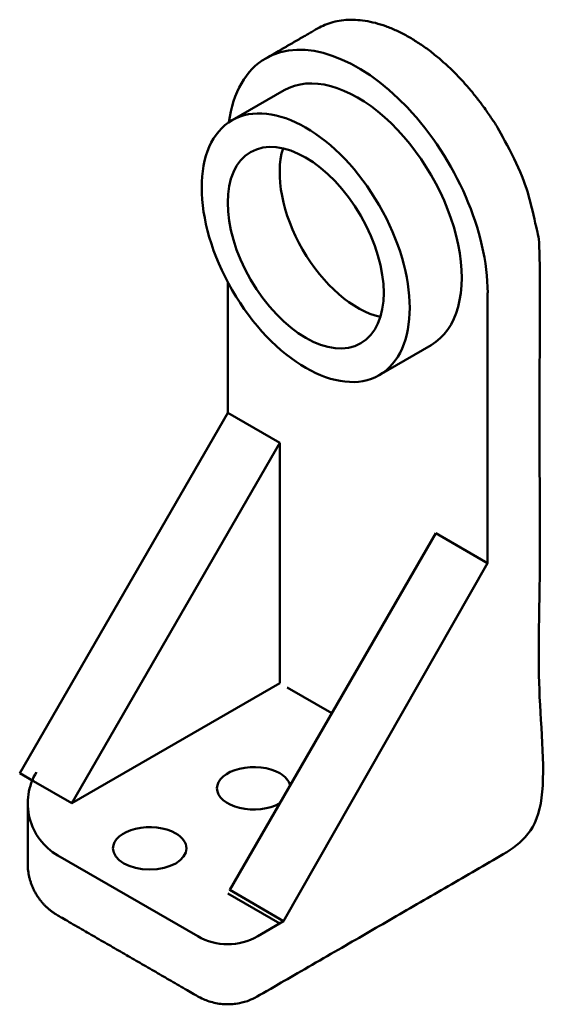
# Model space of a CAD drawing. Units: millimetres. Extents: x 18 to 106, y 44 to 208.
import ezdxf

# ---------------------------------------------------------------- set-up
doc = ezdxf.new("R2010")
doc.units = ezdxf.units.MM
doc.header["$MEASUREMENT"] = 0
doc.layers.add('M-OUTL', color=7, linetype='Continuous', lineweight=50)

msp = doc.modelspace()

# ---------------------------------------------------------------- linework, layer by layer
at = {"layer": 'M-OUTL'}
for p, q in [((61.84, 196.21), (53.18, 191.21)), ((52.44, 142.5), (52.44, 164.27)), ((95.74, 117.5), (95.74, 162.5)), ((77.67, 148.78), (86.33, 153.78)), ((52.44, 142.5), (17.8, 82.5)), ((61.1, 137.5), (52.44, 142.5)), ((61.1, 137.5), (26.46, 77.5)), ((61.1, 97.5), (61.1, 137.5)), ((95.74, 117.5), (95.74, 117.5)), ((26.46, 77.5), (61.1, 97.5)), ((20.12, 81.16), (17.8, 82.5)), ((26.46, 77.5), (20.12, 81.16)), ((61.1, 57.5), (52.44, 62.5))]:
    msp.add_line(p, q, dxfattribs=at)
msp.add_lwpolyline([(87.08, 122.5), (52.77, 63.07), (61.76, 57.88), (95.74, 117.5)], close=True, dxfattribs=at)
msp.add_lwpolyline([(62.32, 96.79), (69.76, 92.5)], dxfattribs=at)
msp.add_lwpolyline([(61.76, 57.88), (57.44, 55.38, -0.267949), (47.44, 55.38), (24.13, 68.84, -0.421376), (20.6, 82.71)], format="xyb", dxfattribs=at)
for centre, major_axis, start_param, end_param in [((74.09, 175), (15.31, -26.52), 0.785398, 3.141593), ((74.09, 175), (15.31, -26.52), 3.141593, 3.786395), ((74.09, 175), (12.25, -21.21), 6.283185, 9.424778), ((82.75, 180), (15.31, -26.52), 10.068279, 10.069581), ((74.09, 175), (9.19, -15.91), 3.632475, 5.792303), ((82.75, 180), (15.31, -26.52), 5.638383, 5.639684), ((56.77, 80), (6.12, 0), 0.785398, 3.141593), ((56.77, 80), (6.12, 0), 0.141897, 0.785398), ((56.77, 80), (6.12, 0), 3.141593, 5.497787), ((39.45, 70), (6.12, 0), 0.785398, 3.141593), ((39.45, 70), (6.12, 0), 0, 0.785398), ((39.45, 70), (6.12, 0), 3.141593, 6.283185)]:
    msp.add_ellipse(centre, major_axis=major_axis, ratio=0.57735, start_param=start_param, end_param=end_param, dxfattribs=at)
for major_axis in [(12.25, -21.21), (9.19, -15.91)]:
    msp.add_ellipse((65.43, 170), major_axis=major_axis, ratio=0.57735, dxfattribs=at)
msp.add_rational_spline([(19.13, 77.5), (19.13, 72.5), (19.13, 67.5), (19.13, 61.72), (24.13, 58.84), (35.79, 52.11), (47.44, 45.38), (52.44, 42.5), (57.44, 45.38), (80.92, 58.94), (104.4, 72.5), (104.4, 120), (104.4, 167.5), (104.4, 184.2), (91.03, 198.31), (77.67, 212.42), (67.44, 206.51), (63.11, 204.01), (58.78, 201.51)], [1, 1, 1, 0.866025403784, 1, 1, 1, 0.866025403784, 1, 1, 1, 1, 1, 0.831469612303, 1, 0.831469612303, 1, 1, 1], degree=2, knots=[0, 0, 0, 1, 1, 2.047198, 2.047198, 3.047198, 3.047198, 4.094395, 4.094395, 5.094395, 5.094395, 6.094395, 6.094395, 7.272492, 7.272492, 8.45059, 8.45059, 9.45059, 9.45059, 9.45059], dxfattribs=at)

doc.saveas('drawing.dxf')
